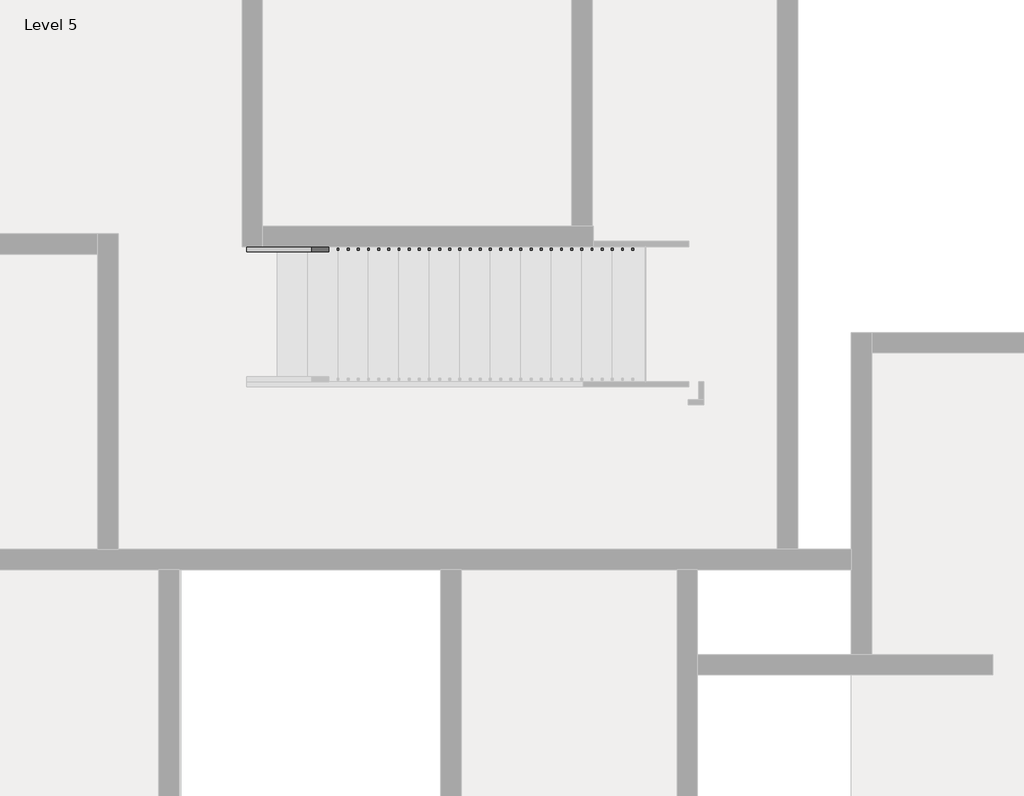
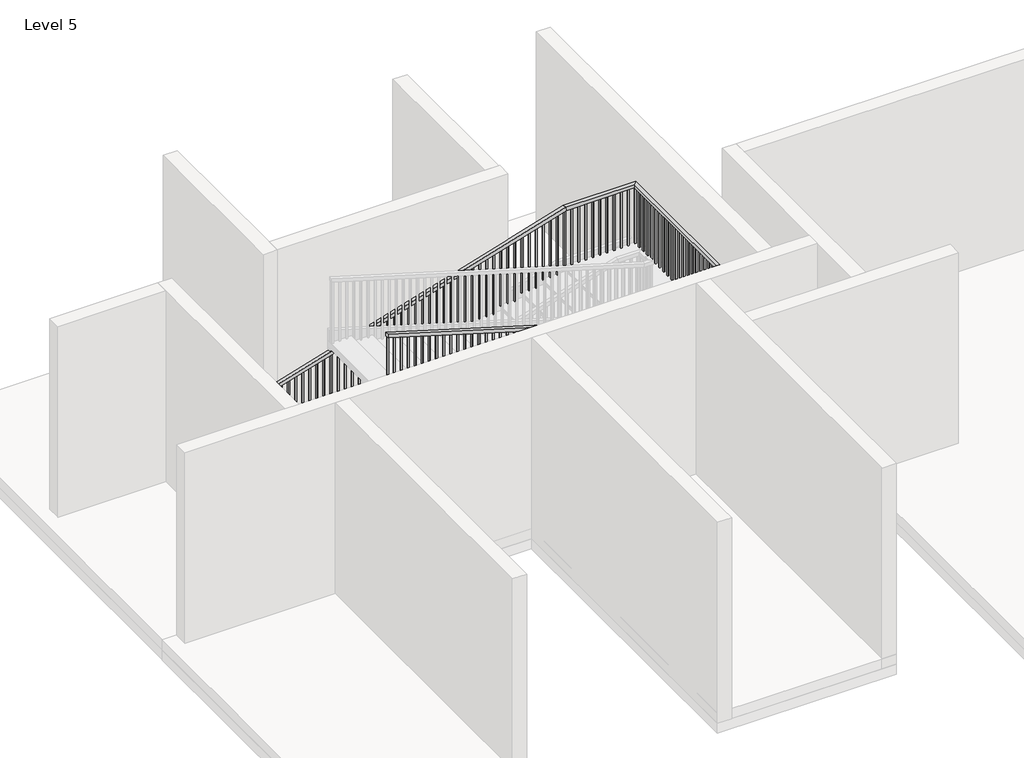
# One storey, part 10 of 14: 1 railing.
"""IFC4 building model written with IfcOpenShell, lengths in millimetres."""

from ifc_helpers import new_model, si_unit, frame, origin, place, context, project, spatial, polyline, outline, extrude, faceted_brep, element, save

model = new_model("IFC4")

# Units and contexts
model_context = context("Model", 3, world=origin())
ifc_project = project(units=[si_unit("LENGTHUNIT", "METRE", prefix="MILLI")], contexts=[model_context])

# Site, building, storey
site = spatial("IfcSite", under=ifc_project)
building = spatial("IfcBuilding", under=site)
storey = spatial("IfcBuildingStorey", under=building, Name="Level 5", Elevation=12192.0)

# Railing
placement = place(None, origin())
element("IfcRailing", 1, ObjectType="Handrail - Rectangular", at=placement, inside=storey, context=model_context, shape_type="SolidModel", body=[
    faceted_brep([(-5254.0891351, 12506.0715905, 13197.84), (-5254.0891351, 12506.0715905, 13144.8032429), (-5254.0891351, 12455.2715905, 13144.8032429), (-5254.0891351, 12455.2715905, 13197.84), (-986.8891351, 12506.0715905, 14478.0), (-979.4332782, 12506.0715905, 14427.2), (-979.4332782, 12455.2715905, 14427.2), (-986.8891351, 12455.2715905, 14478.0), (54.5108649, 12506.0715905, 14478.0), (54.5108649, 12506.0715905, 14427.2), (3.7108649, 12455.2715905, 14427.2), (3.7108649, 12455.2715905, 14478.0), (54.5108649, 9478.4949943, 14478.0), (54.5108649, 9478.4949943, 14427.2), (3.7108649, 9529.2949943, 14427.2), (3.7108649, 9529.2949943, 14478.0), (-682.0891351, 9478.4949943, 14478.0), (-689.544992, 9478.4949943, 14427.2), (-689.544992, 9529.2949943, 14427.2), (-682.0891351, 9529.2949943, 14478.0), (-5254.0891351, 9478.4949943, 15849.6), (-5254.0891351, 9529.2949943, 15849.6), (-5254.0891351, 9529.2949943, 15796.5632429), (-5254.0891351, 9478.4949943, 15796.5632429)], [[[0, 1, 2, 3]], [[1, 0, 4, 5]], [[2, 1, 5, 6]], [[3, 2, 6, 7]], [[0, 3, 7, 4]], [[5, 4, 8, 9]], [[6, 5, 9, 10]], [[7, 6, 10, 11]], [[4, 7, 11, 8]], [[9, 8, 12, 13]], [[10, 9, 13, 14]], [[11, 10, 14, 15]], [[8, 11, 15, 12]], [[13, 12, 16, 17]], [[14, 13, 17, 18]], [[15, 14, 18, 19]], [[12, 15, 19, 16]], [[20, 21, 22, 23]], [[17, 16, 20, 23]], [[18, 17, 23, 22]], [[19, 18, 22, 21]], [[16, 19, 21, 20]]]),
    extrude(outline(polyline([(15768.9407429, -5162.0141351), (14843.76, -5162.0141351), (14843.76, -5142.9641351), (15763.2257429, -5142.9641351), (15768.9407429, -5162.0141351)])), frame((0.0, 9494.3699943, 0.0), z_axis=(0.0, 1.0, 0.0), x_axis=(0.0, 0.0, 1.0)), (0.0, 0.0, 1.0), 19.05),
    extrude(outline(polyline([(15738.4607429, -5060.4141351), (14843.76, -5060.4141351), (14843.76, -5041.3641351), (15732.7457429, -5041.3641351), (15738.4607429, -5060.4141351)])), frame((0.0, 9494.3699943, 0.0), z_axis=(0.0, 1.0, 0.0), x_axis=(0.0, 0.0, 1.0)), (0.0, 0.0, 1.0), 19.05),
    extrude(outline(polyline([(15707.9807429, -4958.8141351), (14843.76, -4958.8141351), (14843.76, -4939.7641351), (15702.2657429, -4939.7641351), (15707.9807429, -4958.8141351)])), frame((0.0, 9494.3699943, 0.0), z_axis=(0.0, 1.0, 0.0), x_axis=(0.0, 0.0, 1.0)), (0.0, 0.0, 1.0), 19.05),
    extrude(outline(polyline([(15677.5007429, -4857.2141351), (14752.32, -4857.2141351), (14752.32, -4838.1641351), (15671.7857429, -4838.1641351), (15677.5007429, -4857.2141351)])), frame((0.0, 9494.3699943, 0.0), z_axis=(0.0, 1.0, 0.0), x_axis=(0.0, 0.0, 1.0)), (0.0, 0.0, 1.0), 19.05),
    extrude(outline(polyline([(15647.0207429, -4755.6141351), (14752.32, -4755.6141351), (14752.32, -4736.5641351), (15641.3057429, -4736.5641351), (15647.0207429, -4755.6141351)])), frame((0.0, 9494.3699943, 0.0), z_axis=(0.0, 1.0, 0.0), x_axis=(0.0, 0.0, 1.0)), (0.0, 0.0, 1.0), 19.05),
    extrude(outline(polyline([(15616.5407429, -4654.0141351), (14752.32, -4654.0141351), (14752.32, -4634.9641351), (15610.8257429, -4634.9641351), (15616.5407429, -4654.0141351)])), frame((0.0, 9494.3699943, 0.0), z_axis=(0.0, 1.0, 0.0), x_axis=(0.0, 0.0, 1.0)), (0.0, 0.0, 1.0), 19.05),
    extrude(outline(polyline([(15586.0607429, -4552.4141351), (14660.88, -4552.4141351), (14660.88, -4533.3641351), (15580.3457429, -4533.3641351), (15586.0607429, -4552.4141351)])), frame((0.0, 9494.3699943, 0.0), z_axis=(0.0, 1.0, 0.0), x_axis=(0.0, 0.0, 1.0)), (0.0, 0.0, 1.0), 19.05),
    extrude(outline(polyline([(15555.5807429, -4450.8141351), (14660.88, -4450.8141351), (14660.88, -4431.7641351), (15549.8657429, -4431.7641351), (15555.5807429, -4450.8141351)])), frame((0.0, 9494.3699943, 0.0), z_axis=(0.0, 1.0, 0.0), x_axis=(0.0, 0.0, 1.0)), (0.0, 0.0, 1.0), 19.05),
    extrude(outline(polyline([(15525.1007429, -4349.2141351), (14660.88, -4349.2141351), (14660.88, -4330.1641351), (15519.3857429, -4330.1641351), (15525.1007429, -4349.2141351)])), frame((0.0, 9494.3699943, 0.0), z_axis=(0.0, 1.0, 0.0), x_axis=(0.0, 0.0, 1.0)), (0.0, 0.0, 1.0), 19.05),
    extrude(outline(polyline([(15494.6207429, -4247.6141351), (14569.44, -4247.6141351), (14569.44, -4228.5641351), (15488.9057429, -4228.5641351), (15494.6207429, -4247.6141351)])), frame((0.0, 9494.3699943, 0.0), z_axis=(0.0, 1.0, 0.0), x_axis=(0.0, 0.0, 1.0)), (0.0, 0.0, 1.0), 19.05),
    extrude(outline(polyline([(15464.1407429, -4146.0141351), (14569.44, -4146.0141351), (14569.44, -4126.9641351), (15458.4257429, -4126.9641351), (15464.1407429, -4146.0141351)])), frame((0.0, 9494.3699943, 0.0), z_axis=(0.0, 1.0, 0.0), x_axis=(0.0, 0.0, 1.0)), (0.0, 0.0, 1.0), 19.05),
    extrude(outline(polyline([(15433.6607429, -4044.4141351), (14569.44, -4044.4141351), (14569.44, -4025.3641351), (15427.9457429, -4025.3641351), (15433.6607429, -4044.4141351)])), frame((0.0, 9494.3699943, 0.0), z_axis=(0.0, 1.0, 0.0), x_axis=(0.0, 0.0, 1.0)), (0.0, 0.0, 1.0), 19.05),
    extrude(outline(polyline([(15403.1807429, -3942.8141351), (14478.0, -3942.8141351), (14478.0, -3923.7641351), (15397.4657429, -3923.7641351), (15403.1807429, -3942.8141351)])), frame((0.0, 9494.3699943, 0.0), z_axis=(0.0, 1.0, 0.0), x_axis=(0.0, 0.0, 1.0)), (0.0, 0.0, 1.0), 19.05),
    extrude(outline(polyline([(15372.7007429, -3841.2141351), (14478.0, -3841.2141351), (14478.0, -3822.1641351), (15366.9857429, -3822.1641351), (15372.7007429, -3841.2141351)])), frame((0.0, 9494.3699943, 0.0), z_axis=(0.0, 1.0, 0.0), x_axis=(0.0, 0.0, 1.0)), (0.0, 0.0, 1.0), 19.05),
    extrude(outline(polyline([(15342.2207429, -3739.6141351), (14478.0, -3739.6141351), (14478.0, -3720.5641351), (15336.5057429, -3720.5641351), (15342.2207429, -3739.6141351)])), frame((0.0, 9494.3699943, 0.0), z_axis=(0.0, 1.0, 0.0), x_axis=(0.0, 0.0, 1.0)), (0.0, 0.0, 1.0), 19.05),
    extrude(outline(polyline([(15311.7407429, -3638.0141351), (14386.56, -3638.0141351), (14386.56, -3618.9641351), (15306.0257429, -3618.9641351), (15311.7407429, -3638.0141351)])), frame((0.0, 9494.3699943, 0.0), z_axis=(0.0, 1.0, 0.0), x_axis=(0.0, 0.0, 1.0)), (0.0, 0.0, 1.0), 19.05),
    extrude(outline(polyline([(15281.2607429, -3536.4141351), (14386.56, -3536.4141351), (14386.56, -3517.3641351), (15275.5457429, -3517.3641351), (15281.2607429, -3536.4141351)])), frame((0.0, 9494.3699943, 0.0), z_axis=(0.0, 1.0, 0.0), x_axis=(0.0, 0.0, 1.0)), (0.0, 0.0, 1.0), 19.05),
    extrude(outline(polyline([(15250.7807429, -3434.8141351), (14386.56, -3434.8141351), (14386.56, -3415.7641351), (15245.0657429, -3415.7641351), (15250.7807429, -3434.8141351)])), frame((0.0, 9494.3699943, 0.0), z_axis=(0.0, 1.0, 0.0), x_axis=(0.0, 0.0, 1.0)), (0.0, 0.0, 1.0), 19.05),
    extrude(outline(polyline([(15220.3007429, -3333.2141351), (14295.12, -3333.2141351), (14295.12, -3314.1641351), (15214.5857429, -3314.1641351), (15220.3007429, -3333.2141351)])), frame((0.0, 9494.3699943, 0.0), z_axis=(0.0, 1.0, 0.0), x_axis=(0.0, 0.0, 1.0)), (0.0, 0.0, 1.0), 19.05),
    extrude(outline(polyline([(15189.8207429, -3231.6141351), (14295.12, -3231.6141351), (14295.12, -3212.5641351), (15184.1057429, -3212.5641351), (15189.8207429, -3231.6141351)])), frame((0.0, 9494.3699943, 0.0), z_axis=(0.0, 1.0, 0.0), x_axis=(0.0, 0.0, 1.0)), (0.0, 0.0, 1.0), 19.05),
    extrude(outline(polyline([(15159.3407429, -3130.0141351), (14295.12, -3130.0141351), (14295.12, -3110.9641351), (15153.6257429, -3110.9641351), (15159.3407429, -3130.0141351)])), frame((0.0, 9494.3699943, 0.0), z_axis=(0.0, 1.0, 0.0), x_axis=(0.0, 0.0, 1.0)), (0.0, 0.0, 1.0), 19.05),
    extrude(outline(polyline([(15128.8607429, -3028.4141351), (14203.68, -3028.4141351), (14203.68, -3009.3641351), (15123.1457429, -3009.3641351), (15128.8607429, -3028.4141351)])), frame((0.0, 9494.3699943, 0.0), z_axis=(0.0, 1.0, 0.0), x_axis=(0.0, 0.0, 1.0)), (0.0, 0.0, 1.0), 19.05),
    extrude(outline(polyline([(15098.3807429, -2926.8141351), (14203.68, -2926.8141351), (14203.68, -2907.7641351), (15092.6657429, -2907.7641351), (15098.3807429, -2926.8141351)])), frame((0.0, 9494.3699943, 0.0), z_axis=(0.0, 1.0, 0.0), x_axis=(0.0, 0.0, 1.0)), (0.0, 0.0, 1.0), 19.05),
    extrude(outline(polyline([(15067.9007429, -2825.2141351), (14203.68, -2825.2141351), (14203.68, -2806.1641351), (15062.1857429, -2806.1641351), (15067.9007429, -2825.2141351)])), frame((0.0, 9494.3699943, 0.0), z_axis=(0.0, 1.0, 0.0), x_axis=(0.0, 0.0, 1.0)), (0.0, 0.0, 1.0), 19.05),
    extrude(outline(polyline([(15037.4207429, -2723.6141351), (14112.24, -2723.6141351), (14112.24, -2704.5641351), (15031.7057429, -2704.5641351), (15037.4207429, -2723.6141351)])), frame((0.0, 9494.3699943, 0.0), z_axis=(0.0, 1.0, 0.0), x_axis=(0.0, 0.0, 1.0)), (0.0, 0.0, 1.0), 19.05),
    extrude(outline(polyline([(15006.9407429, -2622.0141351), (14112.24, -2622.0141351), (14112.24, -2602.9641351), (15001.2257429, -2602.9641351), (15006.9407429, -2622.0141351)])), frame((0.0, 9494.3699943, 0.0), z_axis=(0.0, 1.0, 0.0), x_axis=(0.0, 0.0, 1.0)), (0.0, 0.0, 1.0), 19.05),
    extrude(outline(polyline([(14976.4607429, -2520.4141351), (14112.24, -2520.4141351), (14112.24, -2501.3641351), (14970.7457429, -2501.3641351), (14976.4607429, -2520.4141351)])), frame((0.0, 9494.3699943, 0.0), z_axis=(0.0, 1.0, 0.0), x_axis=(0.0, 0.0, 1.0)), (0.0, 0.0, 1.0), 19.05),
    extrude(outline(polyline([(14945.9807429, -2418.8141351), (14020.8, -2418.8141351), (14020.8, -2399.7641351), (14940.2657429, -2399.7641351), (14945.9807429, -2418.8141351)])), frame((0.0, 9494.3699943, 0.0), z_axis=(0.0, 1.0, 0.0), x_axis=(0.0, 0.0, 1.0)), (0.0, 0.0, 1.0), 19.05),
    extrude(outline(polyline([(14915.5007429, -2317.2141351), (14020.8, -2317.2141351), (14020.8, -2298.1641351), (14909.7857429, -2298.1641351), (14915.5007429, -2317.2141351)])), frame((0.0, 9494.3699943, 0.0), z_axis=(0.0, 1.0, 0.0), x_axis=(0.0, 0.0, 1.0)), (0.0, 0.0, 1.0), 19.05),
    extrude(outline(polyline([(14885.0207429, -2215.6141351), (14020.8, -2215.6141351), (14020.8, -2196.5641351), (14879.3057429, -2196.5641351), (14885.0207429, -2215.6141351)])), frame((0.0, 9494.3699943, 0.0), z_axis=(0.0, 1.0, 0.0), x_axis=(0.0, 0.0, 1.0)), (0.0, 0.0, 1.0), 19.05),
    extrude(outline(polyline([(14854.5407429, -2114.0141351), (13929.36, -2114.0141351), (13929.36, -2094.9641351), (14848.8257429, -2094.9641351), (14854.5407429, -2114.0141351)])), frame((0.0, 9494.3699943, 0.0), z_axis=(0.0, 1.0, 0.0), x_axis=(0.0, 0.0, 1.0)), (0.0, 0.0, 1.0), 19.05),
    extrude(outline(polyline([(14824.0607429, -2012.4141351), (13929.36, -2012.4141351), (13929.36, -1993.3641351), (14818.3457429, -1993.3641351), (14824.0607429, -2012.4141351)])), frame((0.0, 9494.3699943, 0.0), z_axis=(0.0, 1.0, 0.0), x_axis=(0.0, 0.0, 1.0)), (0.0, 0.0, 1.0), 19.05),
    extrude(outline(polyline([(14793.5807429, -1910.8141351), (13929.36, -1910.8141351), (13929.36, -1891.7641351), (14787.8657429, -1891.7641351), (14793.5807429, -1910.8141351)])), frame((0.0, 9494.3699943, 0.0), z_axis=(0.0, 1.0, 0.0), x_axis=(0.0, 0.0, 1.0)), (0.0, 0.0, 1.0), 19.05),
    extrude(outline(polyline([(14763.1007429, -1809.2141351), (13837.92, -1809.2141351), (13837.92, -1790.1641351), (14757.3857429, -1790.1641351), (14763.1007429, -1809.2141351)])), frame((0.0, 9494.3699943, 0.0), z_axis=(0.0, 1.0, 0.0), x_axis=(0.0, 0.0, 1.0)), (0.0, 0.0, 1.0), 19.05),
    extrude(outline(polyline([(14732.6207429, -1707.6141351), (13837.92, -1707.6141351), (13837.92, -1688.5641351), (14726.9057429, -1688.5641351), (14732.6207429, -1707.6141351)])), frame((0.0, 9494.3699943, 0.0), z_axis=(0.0, 1.0, 0.0), x_axis=(0.0, 0.0, 1.0)), (0.0, 0.0, 1.0), 19.05),
    extrude(outline(polyline([(14702.1407429, -1606.0141351), (13837.92, -1606.0141351), (13837.92, -1586.9641351), (14696.4257429, -1586.9641351), (14702.1407429, -1606.0141351)])), frame((0.0, 9494.3699943, 0.0), z_axis=(0.0, 1.0, 0.0), x_axis=(0.0, 0.0, 1.0)), (0.0, 0.0, 1.0), 19.05),
    extrude(outline(polyline([(14671.6607429, -1504.4141351), (13746.48, -1504.4141351), (13746.48, -1485.3641351), (14665.9457429, -1485.3641351), (14671.6607429, -1504.4141351)])), frame((0.0, 9494.3699943, 0.0), z_axis=(0.0, 1.0, 0.0), x_axis=(0.0, 0.0, 1.0)), (0.0, 0.0, 1.0), 19.05),
    extrude(outline(polyline([(14641.1807429, -1402.8141351), (13746.48, -1402.8141351), (13746.48, -1383.7641351), (14635.4657429, -1383.7641351), (14641.1807429, -1402.8141351)])), frame((0.0, 9494.3699943, 0.0), z_axis=(0.0, 1.0, 0.0), x_axis=(0.0, 0.0, 1.0)), (0.0, 0.0, 1.0), 19.05),
    extrude(outline(polyline([(14610.7007429, -1301.2141351), (13746.48, -1301.2141351), (13746.48, -1282.1641351), (14604.9857429, -1282.1641351), (14610.7007429, -1301.2141351)])), frame((0.0, 9494.3699943, 0.0), z_axis=(0.0, 1.0, 0.0), x_axis=(0.0, 0.0, 1.0)), (0.0, 0.0, 1.0), 19.05),
    extrude(outline(polyline([(14580.2207429, -1199.6141351), (13655.04, -1199.6141351), (13655.04, -1180.5641351), (14574.5057429, -1180.5641351), (14580.2207429, -1199.6141351)])), frame((0.0, 9494.3699943, 0.0), z_axis=(0.0, 1.0, 0.0), x_axis=(0.0, 0.0, 1.0)), (0.0, 0.0, 1.0), 19.05),
    extrude(outline(polyline([(14549.7407429, -1098.0141351), (13655.04, -1098.0141351), (13655.04, -1078.9641351), (14544.0257429, -1078.9641351), (14549.7407429, -1098.0141351)])), frame((0.0, 9494.3699943, 0.0), z_axis=(0.0, 1.0, 0.0), x_axis=(0.0, 0.0, 1.0)), (0.0, 0.0, 1.0), 19.05),
    extrude(outline(polyline([(14519.2607429, -996.4141351), (13655.04, -996.4141351), (13655.04, -977.3641351), (14513.5457429, -977.3641351), (14519.2607429, -996.4141351)])), frame((0.0, 9494.3699943, 0.0), z_axis=(0.0, 1.0, 0.0), x_axis=(0.0, 0.0, 1.0)), (0.0, 0.0, 1.0), 19.05),
    extrude(outline(polyline([(14488.7807429, -894.8141351), (13563.6, -894.8141351), (13563.6, -875.7641351), (14483.0657429, -875.7641351), (14488.7807429, -894.8141351)])), frame((0.0, 9494.3699943, 0.0), z_axis=(0.0, 1.0, 0.0), x_axis=(0.0, 0.0, 1.0)), (0.0, 0.0, 1.0), 19.05),
    extrude(outline(polyline([(14458.3007429, -793.2141351), (13563.6, -793.2141351), (13563.6, -774.1641351), (14452.5857429, -774.1641351), (14458.3007429, -793.2141351)])), frame((0.0, 9494.3699943, 0.0), z_axis=(0.0, 1.0, 0.0), x_axis=(0.0, 0.0, 1.0)), (0.0, 0.0, 1.0), 19.05),
    extrude(outline(polyline([(-672.5641351, 9494.3699943), (-691.6141351, 9494.3699943), (-691.6141351, 9513.4199943), (-672.5641351, 9513.4199943), (-672.5641351, 9494.3699943)])), frame((0.0, 0.0, 13563.6), z_axis=(0.0, 0.0, 1.0), x_axis=(1.0, 0.0, 0.0)), (0.0, 0.0, 1.0), 863.6),
    extrude(outline(polyline([(-570.9641351, 9494.3699943), (-590.0141351, 9494.3699943), (-590.0141351, 9513.4199943), (-570.9641351, 9513.4199943), (-570.9641351, 9494.3699943)])), frame((0.0, 0.0, 13563.6), z_axis=(0.0, 0.0, 1.0), x_axis=(1.0, 0.0, 0.0)), (0.0, 0.0, 1.0), 863.6),
    extrude(outline(polyline([(-469.3641351, 9494.3699943), (-488.4141351, 9494.3699943), (-488.4141351, 9513.4199943), (-469.3641351, 9513.4199943), (-469.3641351, 9494.3699943)])), frame((0.0, 0.0, 13563.6), z_axis=(0.0, 0.0, 1.0), x_axis=(1.0, 0.0, 0.0)), (0.0, 0.0, 1.0), 863.6),
    extrude(outline(polyline([(-367.7641351, 9494.3699943), (-386.8141351, 9494.3699943), (-386.8141351, 9513.4199943), (-367.7641351, 9513.4199943), (-367.7641351, 9494.3699943)])), frame((0.0, 0.0, 13563.6), z_axis=(0.0, 0.0, 1.0), x_axis=(1.0, 0.0, 0.0)), (0.0, 0.0, 1.0), 863.6),
    extrude(outline(polyline([(-266.1641351, 9494.3699943), (-285.2141351, 9494.3699943), (-285.2141351, 9513.4199943), (-266.1641351, 9513.4199943), (-266.1641351, 9494.3699943)])), frame((0.0, 0.0, 13563.6), z_axis=(0.0, 0.0, 1.0), x_axis=(1.0, 0.0, 0.0)), (0.0, 0.0, 1.0), 863.6),
    extrude(outline(polyline([(-164.5641351, 9494.3699943), (-183.6141351, 9494.3699943), (-183.6141351, 9513.4199943), (-164.5641351, 9513.4199943), (-164.5641351, 9494.3699943)])), frame((0.0, 0.0, 13563.6), z_axis=(0.0, 0.0, 1.0), x_axis=(1.0, 0.0, 0.0)), (0.0, 0.0, 1.0), 863.6),
    extrude(outline(polyline([(-62.9641351, 9494.3699943), (-82.0141351, 9494.3699943), (-82.0141351, 9513.4199943), (-62.9641351, 9513.4199943), (-62.9641351, 9494.3699943)])), frame((0.0, 0.0, 13563.6), z_axis=(0.0, 0.0, 1.0), x_axis=(1.0, 0.0, 0.0)), (0.0, 0.0, 1.0), 863.6),
    extrude(outline(polyline([(38.6358649, 9543.7965905), (38.6358649, 9524.7465905), (19.5858649, 9524.7465905), (19.5858649, 9543.7965905), (38.6358649, 9543.7965905)])), frame((0.0, 0.0, 13563.6), z_axis=(0.0, 0.0, 1.0), x_axis=(1.0, 0.0, 0.0)), (0.0, 0.0, 1.0), 863.6),
    extrude(outline(polyline([(38.6358649, 9645.3965905), (38.6358649, 9626.3465905), (19.5858649, 9626.3465905), (19.5858649, 9645.3965905), (38.6358649, 9645.3965905)])), frame((0.0, 0.0, 13563.6), z_axis=(0.0, 0.0, 1.0), x_axis=(1.0, 0.0, 0.0)), (0.0, 0.0, 1.0), 863.6),
    extrude(outline(polyline([(38.6358649, 9746.9965905), (38.6358649, 9727.9465905), (19.5858649, 9727.9465905), (19.5858649, 9746.9965905), (38.6358649, 9746.9965905)])), frame((0.0, 0.0, 13563.6), z_axis=(0.0, 0.0, 1.0), x_axis=(1.0, 0.0, 0.0)), (0.0, 0.0, 1.0), 863.6),
    extrude(outline(polyline([(38.6358649, 9848.5965905), (38.6358649, 9829.5465905), (19.5858649, 9829.5465905), (19.5858649, 9848.5965905), (38.6358649, 9848.5965905)])), frame((0.0, 0.0, 13563.6), z_axis=(0.0, 0.0, 1.0), x_axis=(1.0, 0.0, 0.0)), (0.0, 0.0, 1.0), 863.6),
    extrude(outline(polyline([(38.6358649, 9950.1965905), (38.6358649, 9931.1465905), (19.5858649, 9931.1465905), (19.5858649, 9950.1965905), (38.6358649, 9950.1965905)])), frame((0.0, 0.0, 13563.6), z_axis=(0.0, 0.0, 1.0), x_axis=(1.0, 0.0, 0.0)), (0.0, 0.0, 1.0), 863.6),
    extrude(outline(polyline([(38.6358649, 10051.7965905), (38.6358649, 10032.7465905), (19.5858649, 10032.7465905), (19.5858649, 10051.7965905), (38.6358649, 10051.7965905)])), frame((0.0, 0.0, 13563.6), z_axis=(0.0, 0.0, 1.0), x_axis=(1.0, 0.0, 0.0)), (0.0, 0.0, 1.0), 863.6),
    extrude(outline(polyline([(38.6358649, 10153.3965905), (38.6358649, 10134.3465905), (19.5858649, 10134.3465905), (19.5858649, 10153.3965905), (38.6358649, 10153.3965905)])), frame((0.0, 0.0, 13563.6), z_axis=(0.0, 0.0, 1.0), x_axis=(1.0, 0.0, 0.0)), (0.0, 0.0, 1.0), 863.6),
    extrude(outline(polyline([(38.6358649, 10254.9965905), (38.6358649, 10235.9465905), (19.5858649, 10235.9465905), (19.5858649, 10254.9965905), (38.6358649, 10254.9965905)])), frame((0.0, 0.0, 13563.6), z_axis=(0.0, 0.0, 1.0), x_axis=(1.0, 0.0, 0.0)), (0.0, 0.0, 1.0), 863.6),
    extrude(outline(polyline([(38.6358649, 10356.5965905), (38.6358649, 10337.5465905), (19.5858649, 10337.5465905), (19.5858649, 10356.5965905), (38.6358649, 10356.5965905)])), frame((0.0, 0.0, 13563.6), z_axis=(0.0, 0.0, 1.0), x_axis=(1.0, 0.0, 0.0)), (0.0, 0.0, 1.0), 863.6),
    extrude(outline(polyline([(38.6358649, 10458.1965905), (38.6358649, 10439.1465905), (19.5858649, 10439.1465905), (19.5858649, 10458.1965905), (38.6358649, 10458.1965905)])), frame((0.0, 0.0, 13563.6), z_axis=(0.0, 0.0, 1.0), x_axis=(1.0, 0.0, 0.0)), (0.0, 0.0, 1.0), 863.6),
    extrude(outline(polyline([(38.6358649, 10559.7965905), (38.6358649, 10540.7465905), (19.5858649, 10540.7465905), (19.5858649, 10559.7965905), (38.6358649, 10559.7965905)])), frame((0.0, 0.0, 13563.6), z_axis=(0.0, 0.0, 1.0), x_axis=(1.0, 0.0, 0.0)), (0.0, 0.0, 1.0), 863.6),
    extrude(outline(polyline([(38.6358649, 10661.3965905), (38.6358649, 10642.3465905), (19.5858649, 10642.3465905), (19.5858649, 10661.3965905), (38.6358649, 10661.3965905)])), frame((0.0, 0.0, 13563.6), z_axis=(0.0, 0.0, 1.0), x_axis=(1.0, 0.0, 0.0)), (0.0, 0.0, 1.0), 863.6),
    extrude(outline(polyline([(38.6358649, 10762.9965905), (38.6358649, 10743.9465905), (19.5858649, 10743.9465905), (19.5858649, 10762.9965905), (38.6358649, 10762.9965905)])), frame((0.0, 0.0, 13563.6), z_axis=(0.0, 0.0, 1.0), x_axis=(1.0, 0.0, 0.0)), (0.0, 0.0, 1.0), 863.6),
    extrude(outline(polyline([(38.6358649, 10864.5965905), (38.6358649, 10845.5465905), (19.5858649, 10845.5465905), (19.5858649, 10864.5965905), (38.6358649, 10864.5965905)])), frame((0.0, 0.0, 13563.6), z_axis=(0.0, 0.0, 1.0), x_axis=(1.0, 0.0, 0.0)), (0.0, 0.0, 1.0), 863.6),
    extrude(outline(polyline([(38.6358649, 10966.1965905), (38.6358649, 10947.1465905), (19.5858649, 10947.1465905), (19.5858649, 10966.1965905), (38.6358649, 10966.1965905)])), frame((0.0, 0.0, 13563.6), z_axis=(0.0, 0.0, 1.0), x_axis=(1.0, 0.0, 0.0)), (0.0, 0.0, 1.0), 863.6),
    extrude(outline(polyline([(38.6358649, 11067.7965905), (38.6358649, 11048.7465905), (19.5858649, 11048.7465905), (19.5858649, 11067.7965905), (38.6358649, 11067.7965905)])), frame((0.0, 0.0, 13563.6), z_axis=(0.0, 0.0, 1.0), x_axis=(1.0, 0.0, 0.0)), (0.0, 0.0, 1.0), 863.6),
    extrude(outline(polyline([(38.6358649, 11169.3965905), (38.6358649, 11150.3465905), (19.5858649, 11150.3465905), (19.5858649, 11169.3965905), (38.6358649, 11169.3965905)])), frame((0.0, 0.0, 13563.6), z_axis=(0.0, 0.0, 1.0), x_axis=(1.0, 0.0, 0.0)), (0.0, 0.0, 1.0), 863.6),
    extrude(outline(polyline([(38.6358649, 11270.9965905), (38.6358649, 11251.9465905), (19.5858649, 11251.9465905), (19.5858649, 11270.9965905), (38.6358649, 11270.9965905)])), frame((0.0, 0.0, 13563.6), z_axis=(0.0, 0.0, 1.0), x_axis=(1.0, 0.0, 0.0)), (0.0, 0.0, 1.0), 863.6),
    extrude(outline(polyline([(38.6358649, 11372.5965905), (38.6358649, 11353.5465905), (19.5858649, 11353.5465905), (19.5858649, 11372.5965905), (38.6358649, 11372.5965905)])), frame((0.0, 0.0, 13563.6), z_axis=(0.0, 0.0, 1.0), x_axis=(1.0, 0.0, 0.0)), (0.0, 0.0, 1.0), 863.6),
    extrude(outline(polyline([(38.6358649, 11474.1965905), (38.6358649, 11455.1465905), (19.5858649, 11455.1465905), (19.5858649, 11474.1965905), (38.6358649, 11474.1965905)])), frame((0.0, 0.0, 13563.6), z_axis=(0.0, 0.0, 1.0), x_axis=(1.0, 0.0, 0.0)), (0.0, 0.0, 1.0), 863.6),
    extrude(outline(polyline([(38.6358649, 11575.7965905), (38.6358649, 11556.7465905), (19.5858649, 11556.7465905), (19.5858649, 11575.7965905), (38.6358649, 11575.7965905)])), frame((0.0, 0.0, 13563.6), z_axis=(0.0, 0.0, 1.0), x_axis=(1.0, 0.0, 0.0)), (0.0, 0.0, 1.0), 863.6),
    extrude(outline(polyline([(38.6358649, 11677.3965905), (38.6358649, 11658.3465905), (19.5858649, 11658.3465905), (19.5858649, 11677.3965905), (38.6358649, 11677.3965905)])), frame((0.0, 0.0, 13563.6), z_axis=(0.0, 0.0, 1.0), x_axis=(1.0, 0.0, 0.0)), (0.0, 0.0, 1.0), 863.6),
    extrude(outline(polyline([(38.6358649, 11778.9965905), (38.6358649, 11759.9465905), (19.5858649, 11759.9465905), (19.5858649, 11778.9965905), (38.6358649, 11778.9965905)])), frame((0.0, 0.0, 13563.6), z_axis=(0.0, 0.0, 1.0), x_axis=(1.0, 0.0, 0.0)), (0.0, 0.0, 1.0), 863.6),
    extrude(outline(polyline([(38.6358649, 11880.5965905), (38.6358649, 11861.5465905), (19.5858649, 11861.5465905), (19.5858649, 11880.5965905), (38.6358649, 11880.5965905)])), frame((0.0, 0.0, 13563.6), z_axis=(0.0, 0.0, 1.0), x_axis=(1.0, 0.0, 0.0)), (0.0, 0.0, 1.0), 863.6),
    extrude(outline(polyline([(38.6358649, 11982.1965905), (38.6358649, 11963.1465905), (19.5858649, 11963.1465905), (19.5858649, 11982.1965905), (38.6358649, 11982.1965905)])), frame((0.0, 0.0, 13563.6), z_axis=(0.0, 0.0, 1.0), x_axis=(1.0, 0.0, 0.0)), (0.0, 0.0, 1.0), 863.6),
    extrude(outline(polyline([(38.6358649, 12083.7965905), (38.6358649, 12064.7465905), (19.5858649, 12064.7465905), (19.5858649, 12083.7965905), (38.6358649, 12083.7965905)])), frame((0.0, 0.0, 13563.6), z_axis=(0.0, 0.0, 1.0), x_axis=(1.0, 0.0, 0.0)), (0.0, 0.0, 1.0), 863.6),
    extrude(outline(polyline([(38.6358649, 12185.3965905), (38.6358649, 12166.3465905), (19.5858649, 12166.3465905), (19.5858649, 12185.3965905), (38.6358649, 12185.3965905)])), frame((0.0, 0.0, 13563.6), z_axis=(0.0, 0.0, 1.0), x_axis=(1.0, 0.0, 0.0)), (0.0, 0.0, 1.0), 863.6),
    extrude(outline(polyline([(38.6358649, 12286.9965905), (38.6358649, 12267.9465905), (19.5858649, 12267.9465905), (19.5858649, 12286.9965905), (38.6358649, 12286.9965905)])), frame((0.0, 0.0, 13563.6), z_axis=(0.0, 0.0, 1.0), x_axis=(1.0, 0.0, 0.0)), (0.0, 0.0, 1.0), 863.6),
    extrude(outline(polyline([(38.6358649, 12388.5965905), (38.6358649, 12369.5465905), (19.5858649, 12369.5465905), (19.5858649, 12388.5965905), (38.6358649, 12388.5965905)])), frame((0.0, 0.0, 13563.6), z_axis=(0.0, 0.0, 1.0), x_axis=(1.0, 0.0, 0.0)), (0.0, 0.0, 1.0), 863.6),
    extrude(outline(polyline([(-82.0141351, 12490.1965905), (-62.9641351, 12490.1965905), (-62.9641351, 12471.1465905), (-82.0141351, 12471.1465905), (-82.0141351, 12490.1965905)])), frame((0.0, 0.0, 13563.6), z_axis=(0.0, 0.0, 1.0), x_axis=(1.0, 0.0, 0.0)), (0.0, 0.0, 1.0), 863.6),
    extrude(outline(polyline([(-183.6141351, 12490.1965905), (-164.5641351, 12490.1965905), (-164.5641351, 12471.1465905), (-183.6141351, 12471.1465905), (-183.6141351, 12490.1965905)])), frame((0.0, 0.0, 13563.6), z_axis=(0.0, 0.0, 1.0), x_axis=(1.0, 0.0, 0.0)), (0.0, 0.0, 1.0), 863.6),
    extrude(outline(polyline([(-285.2141351, 12490.1965905), (-266.1641351, 12490.1965905), (-266.1641351, 12471.1465905), (-285.2141351, 12471.1465905), (-285.2141351, 12490.1965905)])), frame((0.0, 0.0, 13563.6), z_axis=(0.0, 0.0, 1.0), x_axis=(1.0, 0.0, 0.0)), (0.0, 0.0, 1.0), 863.6),
    extrude(outline(polyline([(-386.8141351, 12490.1965905), (-367.7641351, 12490.1965905), (-367.7641351, 12471.1465905), (-386.8141351, 12471.1465905), (-386.8141351, 12490.1965905)])), frame((0.0, 0.0, 13563.6), z_axis=(0.0, 0.0, 1.0), x_axis=(1.0, 0.0, 0.0)), (0.0, 0.0, 1.0), 863.6),
    extrude(outline(polyline([(-488.4141351, 12490.1965905), (-469.3641351, 12490.1965905), (-469.3641351, 12471.1465905), (-488.4141351, 12471.1465905), (-488.4141351, 12490.1965905)])), frame((0.0, 0.0, 13563.6), z_axis=(0.0, 0.0, 1.0), x_axis=(1.0, 0.0, 0.0)), (0.0, 0.0, 1.0), 863.6),
    extrude(outline(polyline([(-590.0141351, 12490.1965905), (-570.9641351, 12490.1965905), (-570.9641351, 12471.1465905), (-590.0141351, 12471.1465905), (-590.0141351, 12490.1965905)])), frame((0.0, 0.0, 13563.6), z_axis=(0.0, 0.0, 1.0), x_axis=(1.0, 0.0, 0.0)), (0.0, 0.0, 1.0), 863.6),
    extrude(outline(polyline([(-691.6141351, 12490.1965905), (-672.5641351, 12490.1965905), (-672.5641351, 12471.1465905), (-691.6141351, 12471.1465905), (-691.6141351, 12490.1965905)])), frame((0.0, 0.0, 13563.6), z_axis=(0.0, 0.0, 1.0), x_axis=(1.0, 0.0, 0.0)), (0.0, 0.0, 1.0), 863.6),
    extrude(outline(polyline([(-793.2141351, 12490.1965905), (-774.1641351, 12490.1965905), (-774.1641351, 12471.1465905), (-793.2141351, 12471.1465905), (-793.2141351, 12490.1965905)])), frame((0.0, 0.0, 13563.6), z_axis=(0.0, 0.0, 1.0), x_axis=(1.0, 0.0, 0.0)), (0.0, 0.0, 1.0), 863.6),
    extrude(outline(polyline([(-894.8141351, 12490.1965905), (-875.7641351, 12490.1965905), (-875.7641351, 12471.1465905), (-894.8141351, 12471.1465905), (-894.8141351, 12490.1965905)])), frame((0.0, 0.0, 13563.6), z_axis=(0.0, 0.0, 1.0), x_axis=(1.0, 0.0, 0.0)), (0.0, 0.0, 1.0), 863.6),
    extrude(outline(polyline([(14422.1057429, -996.4141351), (13563.6, -996.4141351), (13563.6, -977.3641351), (14427.8207429, -977.3641351), (14422.1057429, -996.4141351)])), frame((0.0, 12471.1465905, 0.0), z_axis=(0.0, 1.0, 0.0), x_axis=(0.0, 0.0, 1.0)), (0.0, 0.0, 1.0), 19.05),
    extrude(outline(polyline([(14391.6257429, -1098.0141351), (13472.16, -1098.0141351), (13472.16, -1078.9641351), (14397.3407429, -1078.9641351), (14391.6257429, -1098.0141351)])), frame((0.0, 12471.1465905, 0.0), z_axis=(0.0, 1.0, 0.0), x_axis=(0.0, 0.0, 1.0)), (0.0, 0.0, 1.0), 19.05),
    extrude(outline(polyline([(14361.1457429, -1199.6141351), (13472.16, -1199.6141351), (13472.16, -1180.5641351), (14366.8607429, -1180.5641351), (14361.1457429, -1199.6141351)])), frame((0.0, 12471.1465905, 0.0), z_axis=(0.0, 1.0, 0.0), x_axis=(0.0, 0.0, 1.0)), (0.0, 0.0, 1.0), 19.05),
    extrude(outline(polyline([(14330.6657429, -1301.2141351), (13472.16, -1301.2141351), (13472.16, -1282.1641351), (14336.3807429, -1282.1641351), (14330.6657429, -1301.2141351)])), frame((0.0, 12471.1465905, 0.0), z_axis=(0.0, 1.0, 0.0), x_axis=(0.0, 0.0, 1.0)), (0.0, 0.0, 1.0), 19.05),
    extrude(outline(polyline([(14300.1857429, -1402.8141351), (13380.72, -1402.8141351), (13380.72, -1383.7641351), (14305.9007429, -1383.7641351), (14300.1857429, -1402.8141351)])), frame((0.0, 12471.1465905, 0.0), z_axis=(0.0, 1.0, 0.0), x_axis=(0.0, 0.0, 1.0)), (0.0, 0.0, 1.0), 19.05),
    extrude(outline(polyline([(14269.7057429, -1504.4141351), (13380.72, -1504.4141351), (13380.72, -1485.3641351), (14275.4207429, -1485.3641351), (14269.7057429, -1504.4141351)])), frame((0.0, 12471.1465905, 0.0), z_axis=(0.0, 1.0, 0.0), x_axis=(0.0, 0.0, 1.0)), (0.0, 0.0, 1.0), 19.05),
    extrude(outline(polyline([(14239.2257429, -1606.0141351), (13380.72, -1606.0141351), (13380.72, -1586.9641351), (14244.9407429, -1586.9641351), (14239.2257429, -1606.0141351)])), frame((0.0, 12471.1465905, 0.0), z_axis=(0.0, 1.0, 0.0), x_axis=(0.0, 0.0, 1.0)), (0.0, 0.0, 1.0), 19.05),
    extrude(outline(polyline([(14208.7457429, -1707.6141351), (13289.28, -1707.6141351), (13289.28, -1688.5641351), (14214.4607429, -1688.5641351), (14208.7457429, -1707.6141351)])), frame((0.0, 12471.1465905, 0.0), z_axis=(0.0, 1.0, 0.0), x_axis=(0.0, 0.0, 1.0)), (0.0, 0.0, 1.0), 19.05),
    extrude(outline(polyline([(14178.2657429, -1809.2141351), (13289.28, -1809.2141351), (13289.28, -1790.1641351), (14183.9807429, -1790.1641351), (14178.2657429, -1809.2141351)])), frame((0.0, 12471.1465905, 0.0), z_axis=(0.0, 1.0, 0.0), x_axis=(0.0, 0.0, 1.0)), (0.0, 0.0, 1.0), 19.05),
    extrude(outline(polyline([(14147.7857429, -1910.8141351), (13289.28, -1910.8141351), (13289.28, -1891.7641351), (14153.5007429, -1891.7641351), (14147.7857429, -1910.8141351)])), frame((0.0, 12471.1465905, 0.0), z_axis=(0.0, 1.0, 0.0), x_axis=(0.0, 0.0, 1.0)), (0.0, 0.0, 1.0), 19.05),
    extrude(outline(polyline([(14117.3057429, -2012.4141351), (13197.84, -2012.4141351), (13197.84, -1993.3641351), (14123.0207429, -1993.3641351), (14117.3057429, -2012.4141351)])), frame((0.0, 12471.1465905, 0.0), z_axis=(0.0, 1.0, 0.0), x_axis=(0.0, 0.0, 1.0)), (0.0, 0.0, 1.0), 19.05),
    extrude(outline(polyline([(14086.8257429, -2114.0141351), (13197.84, -2114.0141351), (13197.84, -2094.9641351), (14092.5407429, -2094.9641351), (14086.8257429, -2114.0141351)])), frame((0.0, 12471.1465905, 0.0), z_axis=(0.0, 1.0, 0.0), x_axis=(0.0, 0.0, 1.0)), (0.0, 0.0, 1.0), 19.05),
    extrude(outline(polyline([(14056.3457429, -2215.6141351), (13197.84, -2215.6141351), (13197.84, -2196.5641351), (14062.0607429, -2196.5641351), (14056.3457429, -2215.6141351)])), frame((0.0, 12471.1465905, 0.0), z_axis=(0.0, 1.0, 0.0), x_axis=(0.0, 0.0, 1.0)), (0.0, 0.0, 1.0), 19.05),
    extrude(outline(polyline([(14025.8657429, -2317.2141351), (13106.4, -2317.2141351), (13106.4, -2298.1641351), (14031.5807429, -2298.1641351), (14025.8657429, -2317.2141351)])), frame((0.0, 12471.1465905, 0.0), z_axis=(0.0, 1.0, 0.0), x_axis=(0.0, 0.0, 1.0)), (0.0, 0.0, 1.0), 19.05),
    extrude(outline(polyline([(13995.3857429, -2418.8141351), (13106.4, -2418.8141351), (13106.4, -2399.7641351), (14001.1007429, -2399.7641351), (13995.3857429, -2418.8141351)])), frame((0.0, 12471.1465905, 0.0), z_axis=(0.0, 1.0, 0.0), x_axis=(0.0, 0.0, 1.0)), (0.0, 0.0, 1.0), 19.05),
    extrude(outline(polyline([(13964.9057429, -2520.4141351), (13106.4, -2520.4141351), (13106.4, -2501.3641351), (13970.6207429, -2501.3641351), (13964.9057429, -2520.4141351)])), frame((0.0, 12471.1465905, 0.0), z_axis=(0.0, 1.0, 0.0), x_axis=(0.0, 0.0, 1.0)), (0.0, 0.0, 1.0), 19.05),
    extrude(outline(polyline([(13934.4257429, -2622.0141351), (13014.96, -2622.0141351), (13014.96, -2602.9641351), (13940.1407429, -2602.9641351), (13934.4257429, -2622.0141351)])), frame((0.0, 12471.1465905, 0.0), z_axis=(0.0, 1.0, 0.0), x_axis=(0.0, 0.0, 1.0)), (0.0, 0.0, 1.0), 19.05),
    extrude(outline(polyline([(13903.9457429, -2723.6141351), (13014.96, -2723.6141351), (13014.96, -2704.5641351), (13909.6607429, -2704.5641351), (13903.9457429, -2723.6141351)])), frame((0.0, 12471.1465905, 0.0), z_axis=(0.0, 1.0, 0.0), x_axis=(0.0, 0.0, 1.0)), (0.0, 0.0, 1.0), 19.05),
    extrude(outline(polyline([(13873.4657429, -2825.2141351), (13014.96, -2825.2141351), (13014.96, -2806.1641351), (13879.1807429, -2806.1641351), (13873.4657429, -2825.2141351)])), frame((0.0, 12471.1465905, 0.0), z_axis=(0.0, 1.0, 0.0), x_axis=(0.0, 0.0, 1.0)), (0.0, 0.0, 1.0), 19.05),
    extrude(outline(polyline([(13842.9857429, -2926.8141351), (12923.52, -2926.8141351), (12923.52, -2907.7641351), (13848.7007429, -2907.7641351), (13842.9857429, -2926.8141351)])), frame((0.0, 12471.1465905, 0.0), z_axis=(0.0, 1.0, 0.0), x_axis=(0.0, 0.0, 1.0)), (0.0, 0.0, 1.0), 19.05),
    extrude(outline(polyline([(13812.5057429, -3028.4141351), (12923.52, -3028.4141351), (12923.52, -3009.3641351), (13818.2207429, -3009.3641351), (13812.5057429, -3028.4141351)])), frame((0.0, 12471.1465905, 0.0), z_axis=(0.0, 1.0, 0.0), x_axis=(0.0, 0.0, 1.0)), (0.0, 0.0, 1.0), 19.05),
    extrude(outline(polyline([(13782.0257429, -3130.0141351), (12923.52, -3130.0141351), (12923.52, -3110.9641351), (13787.7407429, -3110.9641351), (13782.0257429, -3130.0141351)])), frame((0.0, 12471.1465905, 0.0), z_axis=(0.0, 1.0, 0.0), x_axis=(0.0, 0.0, 1.0)), (0.0, 0.0, 1.0), 19.05),
    extrude(outline(polyline([(13751.5457429, -3231.6141351), (12832.08, -3231.6141351), (12832.08, -3212.5641351), (13757.2607429, -3212.5641351), (13751.5457429, -3231.6141351)])), frame((0.0, 12471.1465905, 0.0), z_axis=(0.0, 1.0, 0.0), x_axis=(0.0, 0.0, 1.0)), (0.0, 0.0, 1.0), 19.05),
    extrude(outline(polyline([(13721.0657429, -3333.2141351), (12832.08, -3333.2141351), (12832.08, -3314.1641351), (13726.7807429, -3314.1641351), (13721.0657429, -3333.2141351)])), frame((0.0, 12471.1465905, 0.0), z_axis=(0.0, 1.0, 0.0), x_axis=(0.0, 0.0, 1.0)), (0.0, 0.0, 1.0), 19.05),
    extrude(outline(polyline([(13690.5857429, -3434.8141351), (12832.08, -3434.8141351), (12832.08, -3415.7641351), (13696.3007429, -3415.7641351), (13690.5857429, -3434.8141351)])), frame((0.0, 12471.1465905, 0.0), z_axis=(0.0, 1.0, 0.0), x_axis=(0.0, 0.0, 1.0)), (0.0, 0.0, 1.0), 19.05),
    extrude(outline(polyline([(13660.1057429, -3536.4141351), (12740.64, -3536.4141351), (12740.64, -3517.3641351), (13665.8207429, -3517.3641351), (13660.1057429, -3536.4141351)])), frame((0.0, 12471.1465905, 0.0), z_axis=(0.0, 1.0, 0.0), x_axis=(0.0, 0.0, 1.0)), (0.0, 0.0, 1.0), 19.05),
    extrude(outline(polyline([(13629.6257429, -3638.0141351), (12740.64, -3638.0141351), (12740.64, -3618.9641351), (13635.3407429, -3618.9641351), (13629.6257429, -3638.0141351)])), frame((0.0, 12471.1465905, 0.0), z_axis=(0.0, 1.0, 0.0), x_axis=(0.0, 0.0, 1.0)), (0.0, 0.0, 1.0), 19.05),
    extrude(outline(polyline([(13599.1457429, -3739.6141351), (12740.64, -3739.6141351), (12740.64, -3720.5641351), (13604.8607429, -3720.5641351), (13599.1457429, -3739.6141351)])), frame((0.0, 12471.1465905, 0.0), z_axis=(0.0, 1.0, 0.0), x_axis=(0.0, 0.0, 1.0)), (0.0, 0.0, 1.0), 19.05),
    extrude(outline(polyline([(13568.6657429, -3841.2141351), (12649.2, -3841.2141351), (12649.2, -3822.1641351), (13574.3807429, -3822.1641351), (13568.6657429, -3841.2141351)])), frame((0.0, 12471.1465905, 0.0), z_axis=(0.0, 1.0, 0.0), x_axis=(0.0, 0.0, 1.0)), (0.0, 0.0, 1.0), 19.05),
    extrude(outline(polyline([(13538.1857429, -3942.8141351), (12649.2, -3942.8141351), (12649.2, -3923.7641351), (13543.9007429, -3923.7641351), (13538.1857429, -3942.8141351)])), frame((0.0, 12471.1465905, 0.0), z_axis=(0.0, 1.0, 0.0), x_axis=(0.0, 0.0, 1.0)), (0.0, 0.0, 1.0), 19.05),
    extrude(outline(polyline([(13507.7057429, -4044.4141351), (12649.2, -4044.4141351), (12649.2, -4025.3641351), (13513.4207429, -4025.3641351), (13507.7057429, -4044.4141351)])), frame((0.0, 12471.1465905, 0.0), z_axis=(0.0, 1.0, 0.0), x_axis=(0.0, 0.0, 1.0)), (0.0, 0.0, 1.0), 19.05),
    extrude(outline(polyline([(13477.2257429, -4146.0141351), (12557.76, -4146.0141351), (12557.76, -4126.9641351), (13482.9407429, -4126.9641351), (13477.2257429, -4146.0141351)])), frame((0.0, 12471.1465905, 0.0), z_axis=(0.0, 1.0, 0.0), x_axis=(0.0, 0.0, 1.0)), (0.0, 0.0, 1.0), 19.05),
    extrude(outline(polyline([(13446.7457429, -4247.6141351), (12557.76, -4247.6141351), (12557.76, -4228.5641351), (13452.4607429, -4228.5641351), (13446.7457429, -4247.6141351)])), frame((0.0, 12471.1465905, 0.0), z_axis=(0.0, 1.0, 0.0), x_axis=(0.0, 0.0, 1.0)), (0.0, 0.0, 1.0), 19.05),
    extrude(outline(polyline([(13416.2657429, -4349.2141351), (12557.76, -4349.2141351), (12557.76, -4330.1641351), (13421.9807429, -4330.1641351), (13416.2657429, -4349.2141351)])), frame((0.0, 12471.1465905, 0.0), z_axis=(0.0, 1.0, 0.0), x_axis=(0.0, 0.0, 1.0)), (0.0, 0.0, 1.0), 19.05),
    extrude(outline(polyline([(13385.7857429, -4450.8141351), (12466.32, -4450.8141351), (12466.32, -4431.7641351), (13391.5007429, -4431.7641351), (13385.7857429, -4450.8141351)])), frame((0.0, 12471.1465905, 0.0), z_axis=(0.0, 1.0, 0.0), x_axis=(0.0, 0.0, 1.0)), (0.0, 0.0, 1.0), 19.05),
    extrude(outline(polyline([(13355.3057429, -4552.4141351), (12466.32, -4552.4141351), (12466.32, -4533.3641351), (13361.0207429, -4533.3641351), (13355.3057429, -4552.4141351)])), frame((0.0, 12471.1465905, 0.0), z_axis=(0.0, 1.0, 0.0), x_axis=(0.0, 0.0, 1.0)), (0.0, 0.0, 1.0), 19.05),
    extrude(outline(polyline([(13324.8257429, -4654.0141351), (12466.32, -4654.0141351), (12466.32, -4634.9641351), (13330.5407429, -4634.9641351), (13324.8257429, -4654.0141351)])), frame((0.0, 12471.1465905, 0.0), z_axis=(0.0, 1.0, 0.0), x_axis=(0.0, 0.0, 1.0)), (0.0, 0.0, 1.0), 19.05),
    extrude(outline(polyline([(13294.3457429, -4755.6141351), (12374.88, -4755.6141351), (12374.88, -4736.5641351), (13300.0607429, -4736.5641351), (13294.3457429, -4755.6141351)])), frame((0.0, 12471.1465905, 0.0), z_axis=(0.0, 1.0, 0.0), x_axis=(0.0, 0.0, 1.0)), (0.0, 0.0, 1.0), 19.05),
    extrude(outline(polyline([(13263.8657429, -4857.2141351), (12374.88, -4857.2141351), (12374.88, -4838.1641351), (13269.5807429, -4838.1641351), (13263.8657429, -4857.2141351)])), frame((0.0, 12471.1465905, 0.0), z_axis=(0.0, 1.0, 0.0), x_axis=(0.0, 0.0, 1.0)), (0.0, 0.0, 1.0), 19.05),
    extrude(outline(polyline([(13233.3857429, -4958.8141351), (12374.88, -4958.8141351), (12374.88, -4939.7641351), (13239.1007429, -4939.7641351), (13233.3857429, -4958.8141351)])), frame((0.0, 12471.1465905, 0.0), z_axis=(0.0, 1.0, 0.0), x_axis=(0.0, 0.0, 1.0)), (0.0, 0.0, 1.0), 19.05),
    extrude(outline(polyline([(13202.9057429, -5060.4141351), (12283.44, -5060.4141351), (12283.44, -5041.3641351), (13208.6207429, -5041.3641351), (13202.9057429, -5060.4141351)])), frame((0.0, 12471.1465905, 0.0), z_axis=(0.0, 1.0, 0.0), x_axis=(0.0, 0.0, 1.0)), (0.0, 0.0, 1.0), 19.05),
    extrude(outline(polyline([(13172.4257429, -5162.0141351), (12283.44, -5162.0141351), (12283.44, -5142.9641351), (13178.1407429, -5142.9641351), (13172.4257429, -5162.0141351)])), frame((0.0, 12471.1465905, 0.0), z_axis=(0.0, 1.0, 0.0), x_axis=(0.0, 0.0, 1.0)), (0.0, 0.0, 1.0), 19.05),
    extrude(outline(polyline([(38.6358649, 9513.4199943), (38.6358649, 9494.3699943), (19.5858649, 9494.3699943), (19.5858649, 9513.4199943), (38.6358649, 9513.4199943)])), frame((0.0, 0.0, 13563.6), z_axis=(0.0, 0.0, 1.0), x_axis=(1.0, 0.0, 0.0)), (0.0, 0.0, 1.0), 863.6),
    extrude(outline(polyline([(19.5858649, 12490.1965905), (38.6358649, 12490.1965905), (38.6358649, 12471.1465905), (19.5858649, 12471.1465905), (19.5858649, 12490.1965905)])), frame((0.0, 0.0, 13563.6), z_axis=(0.0, 0.0, 1.0), x_axis=(1.0, 0.0, 0.0)), (0.0, 0.0, 1.0), 863.6),
    extrude(outline(polyline([(15796.5632429, -5254.0891351), (14843.76, -5254.0891351), (14843.76, -5235.0391351), (15790.8482429, -5235.0391351), (15796.5632429, -5254.0891351)])), frame((0.0, 9494.3699943, 0.0), z_axis=(0.0, 1.0, 0.0), x_axis=(0.0, 0.0, 1.0)), (0.0, 0.0, 1.0), 19.05),
    extrude(outline(polyline([(13144.8032429, -5254.0891351), (12283.44, -5254.0891351), (12283.44, -5235.0391351), (13150.5182429, -5235.0391351), (13144.8032429, -5254.0891351)])), frame((0.0, 12471.1465905, 0.0), z_axis=(0.0, 1.0, 0.0), x_axis=(0.0, 0.0, 1.0)), (0.0, 0.0, 1.0), 19.05),
])

save(model, "model.ifc")

# Revit data of these elements
# Type "Handrail - Rectangular"
#   Assembly Code = "C2010400"
#   built-in parameter 1008612 = 0.0416667 (stored number, unit not read)
#   built-in parameter 1008611 = 0.0416667 (stored number, unit not read)
#   built-in parameter 1008609 = 0.333333 (stored number, unit not read)
#   built-in parameter 1008604 = 0.166667 (stored number, unit not read)
#   built-in parameter 1008603 = 0.166667 (stored number, unit not read)
#   Railing Height = 3' - 0"
#   built-in parameter 1008630 = 2
#   built-in parameter 1008610 = 2
#   built-in parameter 1008618 = Baluster - Square : 3/4"
# Element 1 (IfcRailing, "Handrail - Rectangular")
#   Phase Created = New Construction
